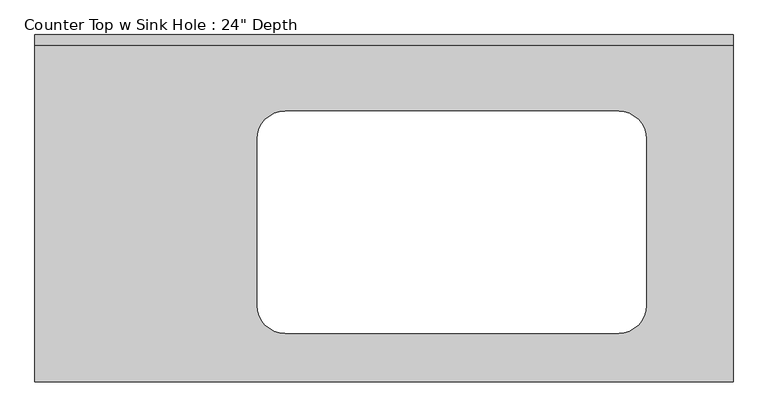
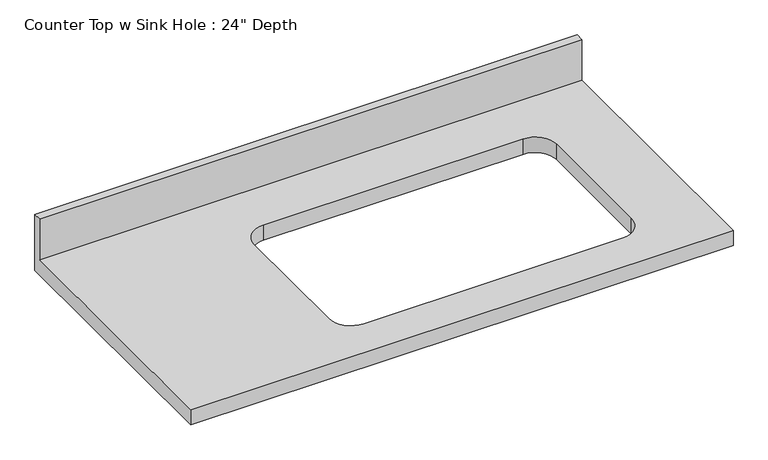
"""IFC4 building model written with IfcOpenShell, lengths in millimetres: furniture geometry."""

from ifc_helpers import new_model, si_unit, frame, origin, place, context, project, spatial, polyline, circle_curve, source, transform, mapped, element, save
from ifc_brep_helpers import plane_surface, revolved_surface, advanced_brep


def furniture_1cc325eb(model_context):
    return source(origin(), model_context, "Body", "AdvancedBrep", [
        advanced_brep(
        [(-1200.4622951, -635.0, 914.4), (75.8877049, -635.0, 914.4), (75.8877049, -19.05, 914.4), (-1200.4622951, -19.05, 914.4), (-743.0967255, -139.7, 914.4), (-133.4967255, -139.7, 914.4), (-82.6967255, -190.5, 914.4), (-82.6967255, -495.3, 914.4), (-133.4967255, -546.1, 914.4), (-743.0967255, -546.1, 914.4), (-793.8967255, -495.3, 914.4), (-793.8967255, -190.5, 914.4), (75.8877049, 0.0, 876.3), (75.8877049, -635.0, 876.3), (-1200.4622951, -635.0, 876.3), (-1200.4622951, 0.0, 876.3), (-133.4967255, -139.7, 876.3), (-743.0967255, -139.7, 876.3), (-793.8967255, -190.5, 876.3), (-793.8967255, -495.3, 876.3), (-743.0967255, -546.1, 876.3), (-133.4967255, -546.1, 876.3), (-82.6967255, -495.3, 876.3), (-82.6967255, -190.5, 876.3), (-1200.4622951, 0.0, 1016.0), (75.8877049, 0.0, 1016.0), (-1200.4622951, -19.05, 1016.0), (75.8877049, -19.05, 1016.0)],
        [
            (0, 1),
            (1, 2),
            (2, 3),
            (3, 0),
            (4, 5),
            (5, 6, circle_curve(frame((-133.4967255, -190.5, 914.4), z_axis=(0.0, 0.0, -1.0), x_axis=(1.0, 0.0, 0.0)), 50.8)),
            (6, 7),
            (7, 8, circle_curve(frame((-133.4967255, -495.3, 914.4), z_axis=(0.0, 0.0, -1.0), x_axis=(1.0, 0.0, 0.0)), 50.8)),
            (8, 9),
            (9, 10, circle_curve(frame((-743.0967255, -495.3, 914.4), z_axis=(0.0, 0.0, -1.0), x_axis=(1.0, 0.0, 0.0)), 50.8)),
            (10, 11),
            (11, 4, circle_curve(frame((-743.0967255, -190.5, 914.4), z_axis=(0.0, 0.0, -1.0), x_axis=(1.0, 0.0, 0.0)), 50.8)),
            (12, 13),
            (13, 14),
            (14, 15),
            (15, 12),
            (16, 17),
            (17, 18, circle_curve(frame((-743.0967255, -190.5, 876.3), z_axis=(0.0, 0.0, 1.0), x_axis=(1.0, 0.0, 0.0)), 50.8)),
            (18, 19),
            (19, 20, circle_curve(frame((-743.0967255, -495.3, 876.3), z_axis=(0.0, 0.0, 1.0), x_axis=(1.0, 0.0, 0.0)), 50.8)),
            (20, 21),
            (21, 22, circle_curve(frame((-133.4967255, -495.3, 876.3), z_axis=(0.0, 0.0, 1.0), x_axis=(1.0, 0.0, 0.0)), 50.8)),
            (22, 23),
            (23, 16, circle_curve(frame((-133.4967255, -190.5, 876.3), z_axis=(0.0, 0.0, 1.0), x_axis=(1.0, 0.0, 0.0)), 50.8)),
            (15, 24),
            (24, 25),
            (25, 12),
            (14, 0),
            (3, 26),
            (26, 24),
            (13, 1),
            (25, 27),
            (27, 2),
            (26, 27),
            (4, 17),
            (16, 5),
            (11, 18),
            (10, 19),
            (9, 20),
            (8, 21),
            (7, 22),
            (6, 23),
        ],
        [
            plane_surface(frame((-1200.4622951, 0.0, 914.4), z_axis=(0.0, 0.0, 1.0), x_axis=(-1.0, 0.0, 0.0))),
            plane_surface(frame((-1200.4622951, 0.0, 876.3), z_axis=(0.0, 0.0, -1.0), x_axis=(1.0, 0.0, 0.0))),
            plane_surface(frame((75.8877049, 0.0, 914.4), z_axis=(0.0, 1.0, 0.0), x_axis=(0.0, 0.0, -1.0))),
            plane_surface(frame((-1200.4622951, 0.0, 914.4), z_axis=(-1.0, 0.0, 0.0), x_axis=(0.0, 0.0, -1.0))),
            plane_surface(frame((-1200.4622951, -635.0, 914.4), z_axis=(0.0, -1.0, 0.0), x_axis=(0.0, 0.0, -1.0))),
            plane_surface(frame((75.8877049, -635.0, 914.4), z_axis=(1.0, 0.0, 0.0), x_axis=(0.0, 0.0, -1.0))),
            plane_surface(frame((-1200.4622951, 0.0, 1016.0), z_axis=(0.0, 0.0, 1.0), x_axis=(0.0, -1.0, 0.0))),
            plane_surface(frame((-1200.4622951, -19.05, 1016.0), z_axis=(0.0, -1.0, 0.0), x_axis=(0.0, 0.0, -1.0))),
            plane_surface(frame((-133.4967255, -139.7, 914.4), z_axis=(0.0, -1.0, 0.0), x_axis=(0.0, 0.0, -1.0))),
            revolved_surface(polyline([(-692.2967255000001, -190.5, 914.4), (-692.2967255000001, -190.5, 876.3)]), (-743.0967255, -190.5, 876.3), (0.0, 0.0, 1.0)),
            plane_surface(frame((-793.8967255, -190.5, 914.4), z_axis=(1.0, 0.0, 0.0), x_axis=(0.0, 0.0, -1.0))),
            revolved_surface(polyline([(-692.2967255000001, -495.3, 914.4), (-692.2967255000001, -495.3, 876.3)]), (-743.0967255, -495.3, 876.3), (0.0, 0.0, 1.0)),
            plane_surface(frame((-743.0967255, -546.1, 914.4), z_axis=(0.0, 1.0, 0.0), x_axis=(0.0, 0.0, -1.0))),
            revolved_surface(polyline([(-82.6967255, -495.3, 914.4), (-82.6967255, -495.3, 876.3)]), (-133.4967255, -495.3, 876.3), (0.0, 0.0, 1.0)),
            plane_surface(frame((-82.6967255, -495.3, 914.4), z_axis=(-1.0, 0.0, 0.0), x_axis=(0.0, 0.0, -1.0))),
            revolved_surface(polyline([(-82.6967255, -190.5, 914.4), (-82.6967255, -190.5, 876.3)]), (-133.4967255, -190.5, 876.3), (0.0, 0.0, 1.0)),
        ],
        [
            (0, [[1, 2, 3, 4], [5, 6, 7, 8, 9, 10, 11, 12]]),
            (1, [[13, 14, 15, 16], [17, 18, 19, 20, 21, 22, 23, 24]]),
            (2, [[-16, 25, 26, 27]]),
            (3, [[-15, 28, -4, 29, 30, -25]]),
            (4, [[-1, -28, -14, 31]]),
            (5, [[-13, -27, 32, 33, -2, -31]]),
            (6, [[-30, 34, -32, -26]]),
            (7, [[-34, -29, -3, -33]]),
            (8, [[35, -17, 36, -5]]),
            (9, [[-35, -12, 37, -18]]),
            (10, [[-37, -11, 38, -19]]),
            (11, [[-38, -10, 39, -20]]),
            (12, [[-39, -9, 40, -21]]),
            (13, [[-40, -8, 41, -22]]),
            (14, [[-41, -7, 42, -23]]),
            (15, [[-36, -24, -42, -6]]),
        ],
    ),
    ])


if __name__ == "__main__":
    model = new_model("IFC4")
    model_context = context("Model", 3, world=origin())
    ifc_project = project(units=[si_unit("LENGTHUNIT", "METRE", prefix="MILLI")], contexts=[model_context])
    site = spatial("IfcSite", under=ifc_project)
    building = spatial("IfcBuilding", under=site)
    placement = place(None, origin())
    furniture_shape = furniture_1cc325eb(model_context)
    element("IfcFurniture", 1, ObjectType="Counter Top w Sink Hole : 24\" Depth", at=placement, inside=building, context=model_context, shape_type="MappedRepresentation", body=[
        mapped(furniture_shape, transform((0.0, 0.0, 0.0), x_axis=(1.0, 0.0, 0.0), y_axis=(0.0, 1.0, 0.0), z_axis=(0.0, 0.0, 1.0))),
    ])
    save(model, "model.ifc")

# Revit data of these elements
# Type "Counter Top w Sink Hole : 24\" Depth"
#   Assembly Code = "C1030400"
#   Counter Thickness = 0' - 1 1/2"
#   Depth = 2' - 1"
#   Height = 3' - 0"
#   Length [instance default] = 8' - 0"
#   Sink Location [instance default] = 2' - 0"
#   Sink Location To Wall [instance default] = 0' - 6"
#   Sink Opening Depth [instance default] = 1' - 3"
#   Sink Opening Width [instance default] = 2' - 3"
#   Counter Top Material = none
#   Default Elevation = 0
# Element 1 (IfcFurniture, "Counter Top w Sink Hole : 24\" Depth")
#   Length = 4' - 2 1/4"
#   Sink Location = 2' - 6.00652"
#   Materials on its faces: "Counter Top"
# Materials
#   "Counter Top": class "Wood", colour RGB 226 177 128, transparency 0
